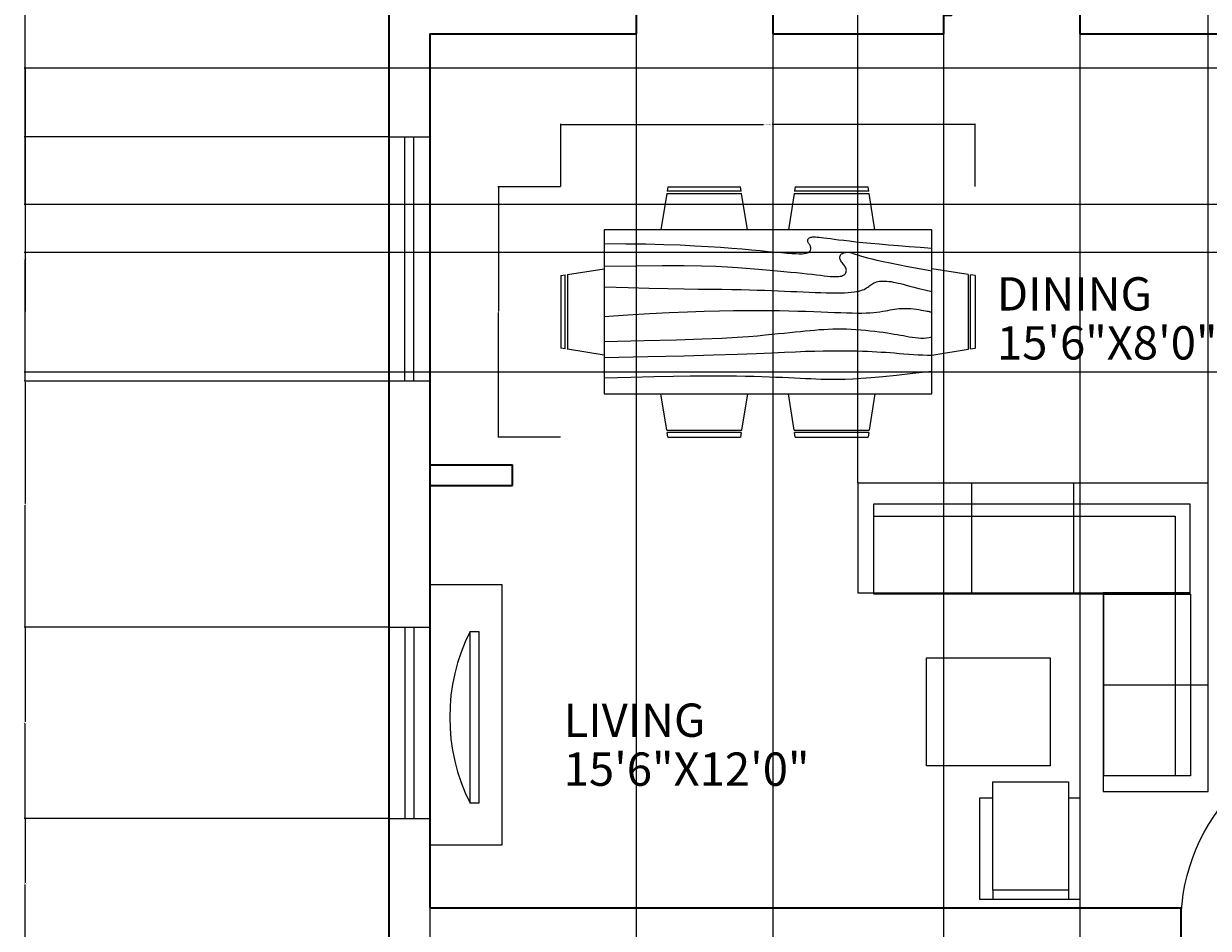
# Model space of a CAD drawing. Units: inches. Extents: x 25018 to 25490, y 41421 to 42101.
# Tile 2 of 5: x 25018 to 25279, y 41707 to 41906. Entities that reach past the tile are written whole.
import ezdxf

# ---------------------------------------------------------------- set-up
doc = ezdxf.new("R2010")
doc.units = ezdxf.units.IN
for name, color, linetype, lineweight in [('A-ANNO-DIMS', 2, 'Continuous', 18), ('A-AREA-IDEN', 7, 'Continuous', 18), ('A-DOOR', 3, 'Continuous', 25), ('A-FURN', 8, 'Continuous', 18), ('A-GLAZ', 4, 'Continuous', 18), ('A-WALL', 7, 'Continuous', 35)]:
    doc.layers.add(name, color=color, linetype=linetype, lineweight=lineweight)
doc.styles.get("Standard").update_dxf_attribs({"font": 'arial.ttf'})
doc.dimstyles.get("Standard").update_dxf_attribs({"dimtxt": 0.18, "dimasz": 0.18, "dimexe": 0.18, "dimexo": 0.0625, "dimgap": 0.09, "dimtad": 0, "dimtih": 1, "dimtoh": 1, "dimdec": 4, "dimzin": 0, "dimdsep": 46, "dimtxsty": 'Standard', "dimcen": 0.09, "dimadec": 0, "dimazin": 0, "dimtfac": 1, "dimtdec": 4, "dimtofl": 0, "dimtmove": 0, "dimatfit": 3, "dimfxl": 1, "dimtolj": 1, "dimtzin": 0, "dimarcsym": 0})

# ---------------------------------------------------------------- blocks, each defined once
blk = doc.blocks.new('*U2')
for p, q in [((0, 0), (0, -100)), ((750, 0), (750, -100))]:
    blk.add_line(p, q)
blk.add_lwpolyline([(0, 0), (0, 750), (43.75, 750), (43.75, 0)], close=True)
blk.add_arc((0, 0), 750, 0, 90)
blk = doc.blocks.new('Dining Set - 36 x 72 in.')
for p, q in [((-22, 27.5), (-22.1562, 26.50042)), ((-5.8416, 26.5), (-22.1534, 26.5)), ((-22, 27.5), (-6, 27.5)), ((-5.8437, 26.49966), (-6, 27.5)), ((6, 27.5), (5.8438, 26.50042)), ((22.1584, 26.5), (5.8466, 26.5)), ((6, 27.5), (22, 27.5)), ((22.1563, 26.49966), (22, 27.5)), ((-22.2343, 26.00059), (-23.4847, 17.99762)), ((-22.2304, 26), (-5.7608, 26)), ((-4.5152, 17.99762), (-5.7655, 25.99926)), ((5.7657, 26.00059), (4.5153, 17.99762)), ((5.7696, 26), (22.2392, 26)), ((23.4848, 17.99762), (22.2345, 25.99926)), ((36, 18), (-36, 18)), ((-36, 18), (-36, -18)), ((36, -18), (36, 18)), ((-45.5, 8), (-44.5004, 8.15617)), ((-45.5, 8), (-45.5, -8)), ((-44.5, -8.15843), (-44.5, 8.15338)), ((-44.0006, 8.23428), (-35.9976, 9.48474)), ((-44, 8.23041), (-44, -8.23915)), ((44.0006, 8.23428), (35.9976, 9.48474)), ((44, 8.23041), (44, -8.23915)), ((44.5, -8.15843), (44.5, 8.15338)), ((45.5, 8), (44.5005, 8.15617)), ((45.5, 8), (45.5, -8)), ((-44.4997, -8.15631), (-45.5, -8)), ((-35.9976, -9.48476), (-43.9993, -8.2345)), ((35.9976, -9.48476), (43.9993, -8.2345)), ((44.4997, -8.15631), (45.5, -8)), ((-36, -18), (36, -18)), ((-22.2343, -26.0006), (-23.4847, -17.99762)), ((-4.5152, -17.99762), (-5.7655, -25.99928)), ((5.7657, -26.0006), (4.5153, -17.99762)), ((23.4848, -17.99762), (22.2345, -25.99928)), ((-22.2304, -26), (-5.7608, -26)), ((5.7696, -26), (22.2392, -26)), ((-22, -27.5), (-22.1562, -26.50044)), ((-5.8416, -26.5), (-22.1534, -26.5)), ((-22, -27.5), (-6, -27.5)), ((-5.8437, -26.49967), (-6, -27.5)), ((6, -27.5), (5.8438, -26.50044)), ((22.1584, -26.5), (5.8466, -26.5)), ((6, -27.5), (22, -27.5)), ((22.1563, -26.49967), (22, -27.5))]:
    blk.add_line(p, q)
for points in [[(-36, 15), (-31.1772, 14.97754), (-26.8079, 14.91406), (-22.8538, 14.81543), (-19.276, 14.6875), (-16.0362, 14.53613), (-13.0957, 14.36718), (-10.4159, 14.18652), (-7.9583, 14), (-5.6904, 13.81315), (-3.6035, 13.63021), (-1.6954, 13.45508), (0.0365, 13.29166), (1.5945, 13.14388), (2.9811, 13.01562), (4.1988, 12.9108), (5.25, 12.83333), (6.1393, 12.78613), (6.8802, 12.76823), (7.4883, 12.77767), (7.9792, 12.8125), (8.3685, 12.87077), (8.6719, 12.95052), (8.9049, 13.0498), (9.0833, 13.16666), (9.2205, 13.29899), (9.3216, 13.44401), (9.3895, 13.59879), (9.4271, 13.76041), (9.4373, 13.92594), (9.4232, 14.09245), (9.3875, 14.257), (9.3333, 14.41666), (9.2638, 14.56917), (9.1836, 14.71484), (9.0975, 14.85465), (9.0104, 14.98958), (8.9272, 15.1206), (8.8529, 15.2487), (8.7922, 15.37483), (8.75, 15.5), (8.7305, 15.62467), (8.7344, 15.74739), (8.7617, 15.86621), (8.8125, 15.97916), (8.8867, 16.08431), (8.9844, 16.17968), (9.1055, 16.26334), (9.25, 16.33333), (9.4189, 16.38802), (9.6172, 16.42708), (9.8506, 16.45052), (10.125, 16.45833), (10.4463, 16.45052), (10.8203, 16.42708), (11.2529, 16.38802), (11.75, 16.33333), (12.3184, 16.26318), (12.9694, 16.17838), (13.7151, 16.07991), (14.5677, 15.96875), (15.5395, 15.84586), (16.6426, 15.71224), (17.8893, 15.56884), (19.2917, 15.41666), (20.859, 15.25667), (22.5879, 15.08984), (24.4721, 14.91715), (26.5052, 14.73958), (28.6809, 14.5581), (30.9929, 14.3737), (33.4347, 14.18733), (36, 14)], [(-36, 10), (-28.9766, 10.14274), (-23.1725, 10.20442), (-18.4241, 10.19775), (-14.5677, 10.13541), (-11.4399, 10.03011), (-8.877, 9.89453), (-6.7154, 9.74137), (-4.7917, 9.58333), (-2.9698, 9.43082), (-1.2246, 9.28515), (0.4415, 9.14534), (2.026, 9.01041), (3.5266, 8.87939), (4.9408, 8.7513), (6.266, 8.62516), (7.5, 8.5), (8.6411, 8.37549), (9.6914, 8.2539), (10.6538, 8.13818), (11.5312, 8.03125), (12.3267, 7.93603), (13.043, 7.85547), (13.6831, 7.79248), (14.25, 7.75), (14.7471, 7.7303), (15.1797, 7.73307), (15.5537, 7.75732), (15.875, 7.80208), (16.1494, 7.86637), (16.3828, 7.94922), (16.5811, 8.04964), (16.75, 8.16666), (16.8944, 8.29915), (17.0143, 8.44531), (17.1089, 8.60319), (17.1771, 8.77083), (17.218, 8.94629), (17.2305, 9.1276), (17.2137, 9.31282), (17.1667, 9.5), (17.0895, 9.6875), (16.987, 9.875), (16.8649, 10.0625), (16.7292, 10.25), (16.5856, 10.4375), (16.4401, 10.625), (16.2985, 10.8125), (16.1667, 11), (16.05, 11.18733), (15.9518, 11.3737), (15.8752, 11.5581), (15.8229, 11.73958), (15.798, 11.91715), (15.8034, 12.08984), (15.842, 12.25667), (15.9167, 12.41666), (16.0295, 12.56836), (16.1784, 12.70833), (16.3605, 12.83268), (16.5729, 12.9375), (16.8127, 13.01888), (17.0768, 13.07291), (17.3625, 13.0957), (17.6667, 13.08333), (17.9894, 13.03312), (18.3418, 12.94726), (18.7382, 12.82918), (19.1927, 12.68229), (19.7195, 12.51001), (20.3327, 12.31575), (21.0465, 12.10294), (21.875, 11.875), (22.8357, 11.63354), (23.959, 11.37304), (25.2786, 11.08618), (26.8282, 10.76562), (28.6414, 10.40405), (30.752, 9.99414), (33.1936, 9.52856), (36, 9)], [(-36, 5.5), (-30.7157, 5.3348), (-26.069, 5.20963), (-21.9946, 5.11767), (-18.4271, 5.05208), (-15.3009, 5.00602), (-12.5508, 4.97265), (-10.1112, 4.94515), (-7.9167, 4.91666), (-5.909, 4.88167), (-4.0586, 4.83984), (-2.3429, 4.79215), (-0.7396, 4.73958), (0.7739, 4.6831), (2.22, 4.6237), (3.6213, 4.56233), (5, 4.5), (6.373, 4.43782), (7.7344, 4.3776), (9.0723, 4.32129), (10.375, 4.27083), (11.6309, 4.22819), (12.8281, 4.19531), (13.9551, 4.17415), (15, 4.16666), (15.954, 4.17448), (16.819, 4.19791), (17.6001, 4.23698), (18.3021, 4.29166), (18.9299, 4.36198), (19.4883, 4.44791), (19.9823, 4.54948), (20.4167, 4.66666), (20.7969, 4.79899), (21.1302, 4.94401), (21.4245, 5.09879), (21.6875, 5.26041), (21.9271, 5.42594), (22.1511, 5.59245), (22.3672, 5.757), (22.5834, 5.91666), (22.8065, 6.06868), (23.0404, 6.21093), (23.2879, 6.34147), (23.5521, 6.45833), (23.8358, 6.55957), (24.142, 6.64323), (24.4735, 6.70735), (24.8334, 6.75), (25.2235, 6.76969), (25.642, 6.76692), (26.0858, 6.74267), (26.5521, 6.69791), (27.0379, 6.63362), (27.5404, 6.55078), (28.0565, 6.45036), (28.5834, 6.33333), (29.1242, 6.19987), (29.7071, 6.04687), (30.3661, 5.87044), (31.1354, 5.66666), (32.0493, 5.43164), (33.142, 5.16146), (34.4475, 4.85221), (36, 4.5)], [(-36, -1), (-30.7915, -0.6591), (-26.0195, -0.38216), (-21.6519, -0.16284), (-17.6563, 0.00521), (-14.0005, 0.12833), (-10.6523, 0.21289), (-7.5796, 0.26522), (-4.75, 0.29166), (-2.134, 0.29793), (0.2878, 0.28711), (2.5317, 0.26163), (4.6146, 0.22396), (6.5529, 0.17651), (8.3633, 0.12174), (10.0623, 0.06209), (11.6667, 0), (13.1899, -0.06201), (14.6341, -0.1211), (15.9982, -0.17432), (17.2813, -0.21875), (18.4823, -0.25147), (19.6003, -0.26953), (20.6343, -0.27002), (21.5834, -0.25), (22.4481, -0.20768), (23.2357, -0.14584), (23.9549, -0.06836), (24.6146, 0.02083), (25.2235, 0.11784), (25.7904, 0.21875), (26.3241, 0.31966), (26.8334, 0.41666), (27.3265, 0.50618), (27.8099, 0.58593), (28.2894, 0.65397), (28.7709, 0.70833), (29.2601, 0.74707), (29.763, 0.76823), (30.2855, 0.76985), (30.8334, 0.75), (31.4088, 0.70784), (31.9994, 0.64713), (32.589, 0.57275), (33.1615, 0.48958), (33.7008, 0.4025), (34.1908, 0.3164), (34.6153, 0.23616), (34.9584, 0.16666), (35.2099, 0.11165), (35.3848, 0.07031), (35.504, 0.04069), (35.5886, 0.02083), (35.6594, 0.00879), (35.7377, 0.0026), (35.8442, 0.00032), (36, 0)], [(-36, -6.5), (-27.1843, -6.31267), (-20.084, -6.1263), (-14.469, -5.9419), (-10.1094, -5.76042), (-6.7752, -5.58285), (-4.2363, -5.41016), (-2.2629, -5.24333), (-0.625, -5.08334), (0.8708, -4.93099), (2.2715, -4.78646), (3.5872, -4.64974), (4.8281, -4.52084), (6.0046, -4.39974), (7.127, -4.28646), (8.2053, -4.18099), (9.25, -4.08334), (10.2705, -3.99382), (11.2734, -3.91407), (12.2647, -3.84603), (13.25, -3.79167), (14.2354, -3.75293), (15.2266, -3.73177), (16.2295, -3.73015), (17.25, -3.75), (18.2912, -3.79248), (19.3451, -3.85547), (20.4009, -3.93604), (21.4479, -4.03125), (22.4754, -4.13819), (23.4727, -4.25391), (24.4289, -4.37549), (25.3334, -4.5), (26.1785, -4.62492), (26.9694, -4.74935), (27.7145, -4.87281), (28.4219, -4.99479), (29.1, -5.11483), (29.7572, -5.23242), (30.4016, -5.34709), (31.0417, -5.45834), (31.6837, -5.56437), (32.3262, -5.65821), (32.9658, -5.73153), (33.599, -5.77604), (34.2224, -5.78345), (34.8327, -5.74545), (35.4264, -5.65373), (36, -5.5)], [(-36, -10), (-26.4022, -9.81299), (-18.4675, -9.62891), (-11.9839, -9.45069), (-6.7396, -9.28125), (-2.5226, -9.12354), (0.8789, -8.98047), (3.6769, -8.85498), (6.0833, -8.75), (8.2767, -8.66765), (10.3021, -8.60677), (12.1712, -8.56543), (13.8958, -8.54167), (15.4876, -8.53353), (16.9583, -8.53907), (18.3197, -8.55632), (19.5834, -8.58334), (20.7616, -8.61841), (21.8685, -8.66081), (22.9188, -8.71004), (23.9271, -8.76563), (24.9081, -8.82707), (25.8763, -8.89388), (26.8465, -8.96558), (27.8334, -9.04167), (28.8474, -9.12118), (29.8828, -9.20117), (30.93, -9.27824), (31.9792, -9.34896), (33.0205, -9.40991), (34.0443, -9.45768), (35.0407, -9.48885), (36, -9.5)], [(-36, -14.5), (-30.0881, -14.33513), (-25.0332, -14.21224), (-20.7312, -14.12647), (-17.0781, -14.07292), (-13.97, -14.04671), (-11.3027, -14.04297), (-8.9724, -14.05681), (-6.875, -14.08334), (-4.9224, -14.11833), (-3.0905, -14.16016), (-1.3709, -14.20785), (0.2448, -14.26042), (1.7647, -14.3169), (3.1973, -14.3763), (4.5507, -14.43767), (5.8333, -14.5), (7.0554, -14.5621), (8.235, -14.62175), (9.3922, -14.67652), (10.5469, -14.72396), (11.7192, -14.76164), (12.929, -14.78711), (14.1965, -14.79794), (15.5417, -14.79167), (16.9933, -14.76424), (18.6152, -14.70508), (20.4804, -14.60197), (22.6615, -14.44271), (25.2312, -14.21509), (28.2624, -13.9069), (31.8277, -13.50594), (36, -13)]]:
    blk.add_lwpolyline(points)
blk = doc.blocks.new('TV-CONSOLE')
for points in [[(0, 57.27), (15.78, 57.27), (15.78, 0), (0, 0)], [(8.85, 46.95), (10.77, 46.95), (10.77, 9.28), (8.85, 9.28)]]:
    blk.add_lwpolyline(points, close=True)
blk.add_arc((46.16, 28.12), 41.8, 153.2115, 206.7885)
blk = doc.blocks.new('*D26')
at = {"layer": 'A-ANNO-DIMS', "color": 0, "lineweight": -2, "transparency": 16777216}
for p, q in [((25136.41, 41870.05), (25136.41, 41883.82)), ((25136.59, 41883.64), (25180.96, 41883.64)), ((25227.23, 41883.64), (25182.86, 41883.64)), ((25227.41, 41870.05), (25227.41, 41883.82))]:
    blk.add_line(p, q, dxfattribs=at)
at = {"layer": 'A-ANNO-DIMS', "color": 0, "transparency": 16777216}
for points in [[(25136.59, 41883.67), (25136.59, 41883.61), (25136.41, 41883.64)], [(25227.23, 41883.67), (25227.23, 41883.61), (25227.41, 41883.64)]]:
    blk.add_solid(points, dxfattribs=at)
at = {"layer": 'Defpoints', "color": 0, "transparency": 16777216}
for p in [(25227.41, 41883.64), (25136.41, 41869.99), (25227.41, 41869.99)]:
    blk.add_point(p, dxfattribs=at)
at = {"layer": 'A-ANNO-DIMS', "color": 0, "transparency": 16777216, "insert": (25181.91, 41883.64), "char_height": 0.18, "attachment_point": 5}
blk.add_mtext('\\A1;DINING SET 91', dxfattribs=at)
blk = doc.blocks.new('*D27')
at = {"layer": 'A-ANNO-DIMS', "color": 0, "lineweight": -2, "transparency": 16777216}
for p, q in [((25136.34, 41869.99), (25122.58, 41869.99)), ((25122.76, 41869.81), (25122.76, 41842.67)), ((25122.76, 41815.17), (25122.76, 41842.31)), ((25136.34, 41814.99), (25122.58, 41814.99))]:
    blk.add_line(p, q, dxfattribs=at)
at = {"layer": 'A-ANNO-DIMS', "color": 0, "transparency": 16777216}
for points in [[(25122.73, 41869.81), (25122.79, 41869.81), (25122.76, 41869.99)], [(25122.73, 41815.17), (25122.79, 41815.17), (25122.76, 41814.99)]]:
    blk.add_solid(points, dxfattribs=at)
at = {"layer": 'Defpoints', "color": 0, "transparency": 16777216}
for p in [(25122.76, 41869.99), (25136.41, 41869.99), (25136.41, 41814.99)]:
    blk.add_point(p, dxfattribs=at)
at = {"layer": 'A-ANNO-DIMS', "color": 0, "transparency": 16777216, "insert": (25122.76, 41842.49), "char_height": 0.18, "attachment_point": 5}
blk.add_mtext('\\A1;55', dxfattribs=at)
blk = doc.blocks.new('*D44')
at = {"layer": 'A-ANNO-DIMS', "color": 0, "lineweight": -2, "transparency": 16777216}
for p, q in [((25098.59, 41731.2), (25018.58, 41731.2)), ((25018.76, 41731.02), (25018.76, 41717.06)), ((25018.76, 41702.73), (25018.76, 41716.69)), ((25098.59, 41702.55), (25018.58, 41702.55))]:
    blk.add_line(p, q, dxfattribs=at)
at = {"layer": 'A-ANNO-DIMS', "color": 0, "transparency": 16777216}
for points in [[(25018.73, 41731.02), (25018.79, 41731.02), (25018.76, 41731.2)], [(25018.73, 41702.73), (25018.79, 41702.73), (25018.76, 41702.55)]]:
    blk.add_solid(points, dxfattribs=at)
at = {"layer": 'Defpoints', "color": 0, "transparency": 16777216}
for p in [(25018.76, 41731.2), (25098.65, 41731.2), (25098.65, 41702.55)]:
    blk.add_point(p, dxfattribs=at)
at = {"layer": 'A-ANNO-DIMS', "color": 0, "transparency": 16777216, "insert": (25018.76, 41716.88), "char_height": 0.18, "attachment_point": 5}
blk.add_mtext('\\A1;28.65', dxfattribs=at)
blk = doc.blocks.new('*D45')
at = {"layer": 'A-ANNO-DIMS', "color": 0, "lineweight": -2, "transparency": 16777216}
for p, q in [((25098.59, 41773.23), (25018.58, 41773.23)), ((25018.76, 41773.05), (25018.76, 41752.4)), ((25018.76, 41731.38), (25018.76, 41752.03)), ((25098.59, 41731.2), (25018.58, 41731.2))]:
    blk.add_line(p, q, dxfattribs=at)
at = {"layer": 'A-ANNO-DIMS', "color": 0, "transparency": 16777216}
for points in [[(25018.73, 41773.05), (25018.79, 41773.05), (25018.76, 41773.23)], [(25018.73, 41731.38), (25018.79, 41731.38), (25018.76, 41731.2)]]:
    blk.add_solid(points, dxfattribs=at)
at = {"layer": 'Defpoints', "color": 0, "transparency": 16777216}
for p in [(25018.76, 41773.23), (25098.65, 41773.23), (25098.65, 41731.2)]:
    blk.add_point(p, dxfattribs=at)
at = {"layer": 'A-ANNO-DIMS', "color": 0, "transparency": 16777216, "insert": (25018.76, 41752.21), "char_height": 0.18, "attachment_point": 5}
blk.add_mtext('\\A1;42.03', dxfattribs=at)
blk = doc.blocks.new('*D46')
at = {"layer": 'A-ANNO-DIMS', "color": 0, "lineweight": -2, "transparency": 16777216}
for p, q in [((25098.59, 41827.23), (25018.58, 41827.23)), ((25018.76, 41827.05), (25018.76, 41800.41)), ((25018.76, 41773.41), (25018.76, 41800.05)), ((25098.59, 41773.23), (25018.58, 41773.23))]:
    blk.add_line(p, q, dxfattribs=at)
at = {"layer": 'A-ANNO-DIMS', "color": 0, "transparency": 16777216}
for points in [[(25018.73, 41827.05), (25018.79, 41827.05), (25018.76, 41827.23)], [(25018.73, 41773.41), (25018.79, 41773.41), (25018.76, 41773.23)]]:
    blk.add_solid(points, dxfattribs=at)
at = {"layer": 'Defpoints', "color": 0, "transparency": 16777216}
for p in [(25018.76, 41827.23), (25098.65, 41827.23), (25098.65, 41773.23)]:
    blk.add_point(p, dxfattribs=at)
at = {"layer": 'A-ANNO-DIMS', "color": 0, "transparency": 16777216, "insert": (25018.76, 41800.23), "char_height": 0.18, "attachment_point": 5}
blk.add_mtext('\\A1;54', dxfattribs=at)
blk = doc.blocks.new('*D47')
at = {"layer": 'A-ANNO-DIMS', "color": 0, "lineweight": -2, "transparency": 16777216}
for p, q in [((25098.59, 41880.94), (25018.58, 41880.94)), ((25018.76, 41880.76), (25018.76, 41854.27)), ((25018.76, 41827.41), (25018.76, 41853.9)), ((25098.59, 41827.23), (25018.58, 41827.23))]:
    blk.add_line(p, q, dxfattribs=at)
at = {"layer": 'A-ANNO-DIMS', "color": 0, "transparency": 16777216}
for points in [[(25018.73, 41880.76), (25018.79, 41880.76), (25018.76, 41880.94)], [(25018.73, 41827.41), (25018.79, 41827.41), (25018.76, 41827.23)]]:
    blk.add_solid(points, dxfattribs=at)
at = {"layer": 'Defpoints', "color": 0, "transparency": 16777216}
for p in [(25018.76, 41880.94), (25098.65, 41880.94), (25098.65, 41827.23)]:
    blk.add_point(p, dxfattribs=at)
at = {"layer": 'A-ANNO-DIMS', "color": 0, "transparency": 16777216, "insert": (25018.76, 41854.09), "char_height": 0.18, "attachment_point": 5}
blk.add_mtext('\\A1;53.71', dxfattribs=at)
blk = doc.blocks.new('*D48')
at = {"layer": 'A-ANNO-DIMS', "color": 0, "lineweight": -2, "transparency": 16777216}
for p, q in [((25107.59, 42013.05), (25018.58, 42013.05)), ((25018.76, 42012.87), (25018.76, 41947.18)), ((25018.76, 41881.12), (25018.76, 41946.81)), ((25098.59, 41880.94), (25018.58, 41880.94))]:
    blk.add_line(p, q, dxfattribs=at)
at = {"layer": 'A-ANNO-DIMS', "color": 0, "transparency": 16777216}
for points in [[(25018.73, 42012.87), (25018.79, 42012.87), (25018.76, 42013.05)], [(25018.73, 41881.12), (25018.79, 41881.12), (25018.76, 41880.94)]]:
    blk.add_solid(points, dxfattribs=at)
at = {"layer": 'Defpoints', "color": 0, "transparency": 16777216}
for p in [(25018.76, 42013.05), (25107.65, 42013.05), (25098.65, 41880.94)]:
    blk.add_point(p, dxfattribs=at)
at = {"layer": 'A-ANNO-DIMS', "color": 0, "transparency": 16777216, "insert": (25018.76, 41946.99), "char_height": 0.18, "attachment_point": 5}
blk.add_mtext('\\A1;132.1', dxfattribs=at)
blk = doc.blocks.new('*D66')
at = {"layer": 'A-ANNO-DIMS', "color": 0, "lineweight": -2, "transparency": 16777216}
for p, q in [((25107.65, 41903.49), (25107.65, 41420.7)), ((25152.99, 41903.49), (25152.99, 41420.7)), ((25107.83, 41420.88), (25129.92, 41420.88)), ((25152.81, 41420.88), (25130.72, 41420.88))]:
    blk.add_line(p, q, dxfattribs=at)
at = {"layer": 'A-ANNO-DIMS', "color": 0, "transparency": 16777216}
for points in [[(25107.83, 41420.91), (25107.83, 41420.85), (25107.65, 41420.88)], [(25152.81, 41420.91), (25152.81, 41420.85), (25152.99, 41420.88)]]:
    blk.add_solid(points, dxfattribs=at)
at = {"layer": 'Defpoints', "color": 0, "transparency": 16777216}
for p in [(25107.65, 41903.55), (25152.99, 41903.55), (25152.99, 41420.88)]:
    blk.add_point(p, dxfattribs=at)
at = {"layer": 'A-ANNO-DIMS', "color": 0, "transparency": 16777216, "insert": (25130.32, 41420.88), "char_height": 0.18, "attachment_point": 5}
blk.add_mtext('\\A1;45.34', dxfattribs=at)
blk = doc.blocks.new('*D67')
at = {"layer": 'A-ANNO-DIMS', "color": 0, "lineweight": -2, "transparency": 16777216}
for p, q in [((25152.99, 41903.49), (25152.99, 41420.7)), ((25182.99, 41903.49), (25182.99, 41420.7)), ((25153.17, 41420.88), (25167.77, 41420.88)), ((25182.81, 41420.88), (25168.21, 41420.88))]:
    blk.add_line(p, q, dxfattribs=at)
at = {"layer": 'A-ANNO-DIMS', "color": 0, "transparency": 16777216}
for points in [[(25153.17, 41420.91), (25153.17, 41420.85), (25152.99, 41420.88)], [(25182.81, 41420.91), (25182.81, 41420.85), (25182.99, 41420.88)]]:
    blk.add_solid(points, dxfattribs=at)
at = {"layer": 'Defpoints', "color": 0, "transparency": 16777216}
for p in [(25152.99, 41903.55), (25182.99, 41903.55), (25182.99, 41420.88)]:
    blk.add_point(p, dxfattribs=at)
at = {"layer": 'A-ANNO-DIMS', "color": 0, "transparency": 16777216, "insert": (25167.99, 41420.88), "char_height": 0.18, "attachment_point": 5}
blk.add_mtext('\\A1;30', dxfattribs=at)
blk = doc.blocks.new('*D68')
at = {"layer": 'A-ANNO-DIMS', "color": 0, "lineweight": -2, "transparency": 16777216}
for p, q in [((25182.99, 41903.49), (25182.99, 41420.7)), ((25220.45, 41903.49), (25220.45, 41420.7)), ((25183.17, 41420.88), (25201.26, 41420.88)), ((25220.27, 41420.88), (25202.18, 41420.88))]:
    blk.add_line(p, q, dxfattribs=at)
at = {"layer": 'A-ANNO-DIMS', "color": 0, "transparency": 16777216}
for points in [[(25183.17, 41420.91), (25183.17, 41420.85), (25182.99, 41420.88)], [(25220.27, 41420.91), (25220.27, 41420.85), (25220.45, 41420.88)]]:
    blk.add_solid(points, dxfattribs=at)
at = {"layer": 'Defpoints', "color": 0, "transparency": 16777216}
for p in [(25182.99, 41903.55), (25220.45, 41903.55), (25220.45, 41420.88)]:
    blk.add_point(p, dxfattribs=at)
at = {"layer": 'A-ANNO-DIMS', "color": 0, "transparency": 16777216, "insert": (25201.72, 41420.88), "char_height": 0.18, "attachment_point": 5}
blk.add_mtext('\\A1;37.464', dxfattribs=at)
blk = doc.blocks.new('*D69')
at = {"layer": 'A-ANNO-DIMS', "color": 0, "lineweight": -2, "transparency": 16777216}
for p, q in [((25220.45, 41903.49), (25220.45, 41420.7)), ((25250.45, 41903.49), (25250.45, 41420.7)), ((25220.63, 41420.88), (25235.23, 41420.88)), ((25250.27, 41420.88), (25235.67, 41420.88))]:
    blk.add_line(p, q, dxfattribs=at)
at = {"layer": 'A-ANNO-DIMS', "color": 0, "transparency": 16777216}
for points in [[(25220.63, 41420.91), (25220.63, 41420.85), (25220.45, 41420.88)], [(25250.27, 41420.91), (25250.27, 41420.85), (25250.45, 41420.88)]]:
    blk.add_solid(points, dxfattribs=at)
at = {"layer": 'Defpoints', "color": 0, "transparency": 16777216}
for p in [(25220.45, 41903.55), (25250.45, 41903.55), (25250.45, 41420.88)]:
    blk.add_point(p, dxfattribs=at)
at = {"layer": 'A-ANNO-DIMS', "color": 0, "transparency": 16777216, "insert": (25235.45, 41420.88), "char_height": 0.18, "attachment_point": 5}
blk.add_mtext('\\A1;30', dxfattribs=at)
blk = doc.blocks.new('*D70')
at = {"layer": 'A-ANNO-DIMS', "color": 0, "lineweight": -2, "transparency": 16777216}
for p, q in [((25250.45, 41903.49), (25250.45, 41420.7)), ((25302.95, 41903.49), (25302.95, 41420.7)), ((25250.63, 41420.88), (25276.38, 41420.88)), ((25302.77, 41420.88), (25277.03, 41420.88))]:
    blk.add_line(p, q, dxfattribs=at)
at = {"layer": 'A-ANNO-DIMS', "color": 0, "transparency": 16777216}
for points in [[(25250.63, 41420.91), (25250.63, 41420.85), (25250.45, 41420.88)], [(25302.77, 41420.91), (25302.77, 41420.85), (25302.95, 41420.88)]]:
    blk.add_solid(points, dxfattribs=at)
at = {"layer": 'Defpoints', "color": 0, "transparency": 16777216}
for p in [(25250.45, 41903.55), (25302.95, 41903.55), (25302.95, 41420.88)]:
    blk.add_point(p, dxfattribs=at)
at = {"layer": 'A-ANNO-DIMS', "color": 0, "transparency": 16777216, "insert": (25276.7, 41420.88), "char_height": 0.18, "attachment_point": 5}
blk.add_mtext('\\A1;52.5', dxfattribs=at)
blk = doc.blocks.new('*D72')
at = {"layer": 'A-ANNO-DIMS', "color": 0, "lineweight": -2, "transparency": 16777216}
for p, q in [((25338.89, 41896.05), (25018.58, 41896.05)), ((25018.76, 41895.87), (25018.76, 41881.23)), ((25018.76, 41866.23), (25018.76, 41880.87)), ((25338.89, 41866.05), (25018.58, 41866.05))]:
    blk.add_line(p, q, dxfattribs=at)
at = {"layer": 'A-ANNO-DIMS', "color": 0, "transparency": 16777216}
for points in [[(25018.73, 41895.87), (25018.79, 41895.87), (25018.76, 41896.05)], [(25018.73, 41866.23), (25018.79, 41866.23), (25018.76, 41866.05)]]:
    blk.add_solid(points, dxfattribs=at)
at = {"layer": 'Defpoints', "color": 0, "transparency": 16777216}
for p in [(25018.76, 41896.05), (25338.95, 41896.05), (25338.95, 41866.05)]:
    blk.add_point(p, dxfattribs=at)
at = {"layer": 'A-ANNO-DIMS', "color": 0, "transparency": 16777216, "insert": (25018.76, 41881.05), "char_height": 0.18, "attachment_point": 5}
blk.add_mtext('\\A1;30', dxfattribs=at)
blk = doc.blocks.new('*D73')
at = {"layer": 'A-ANNO-DIMS', "color": 0, "lineweight": -2, "transparency": 16777216}
for p, q in [((25338.89, 41855.55), (25018.58, 41855.55)), ((25018.76, 41855.37), (25018.76, 41842.58)), ((25018.76, 41829.43), (25018.76, 41842.22)), ((25338.89, 41829.25), (25018.58, 41829.25))]:
    blk.add_line(p, q, dxfattribs=at)
at = {"layer": 'A-ANNO-DIMS', "color": 0, "transparency": 16777216}
for points in [[(25018.73, 41855.37), (25018.79, 41855.37), (25018.76, 41855.55)], [(25018.73, 41829.43), (25018.79, 41829.43), (25018.76, 41829.25)]]:
    blk.add_solid(points, dxfattribs=at)
at = {"layer": 'Defpoints', "color": 0, "transparency": 16777216}
for p in [(25018.76, 41855.55), (25338.95, 41855.55), (25338.95, 41829.25)]:
    blk.add_point(p, dxfattribs=at)
at = {"layer": 'A-ANNO-DIMS', "color": 0, "transparency": 16777216, "insert": (25018.76, 41842.4), "char_height": 0.18, "attachment_point": 5}
blk.add_mtext('\\A1;26.3', dxfattribs=at)
blk = doc.blocks.new('*D75')
at = {"layer": 'A-ANNO-DIMS', "color": 0, "lineweight": -2, "transparency": 16777216}
for p, q in [((25201.64, 41804.94), (25201.64, 42101.23)), ((25201.82, 42101.05), (25239.92, 42101.05)), ((25278.45, 42101.05), (25240.36, 42101.05)), ((25278.63, 41804.94), (25278.63, 42101.23))]:
    blk.add_line(p, q, dxfattribs=at)
at = {"layer": 'A-ANNO-DIMS', "color": 0, "transparency": 16777216}
for points in [[(25201.82, 42101.08), (25201.82, 42101.02), (25201.64, 42101.05)], [(25278.45, 42101.08), (25278.45, 42101.02), (25278.63, 42101.05)]]:
    blk.add_solid(points, dxfattribs=at)
at = {"layer": 'Defpoints', "color": 0, "transparency": 16777216}
for p in [(25278.63, 42101.05), (25201.64, 41804.88), (25278.63, 41804.88)]:
    blk.add_point(p, dxfattribs=at)
at = {"layer": 'A-ANNO-DIMS', "color": 0, "transparency": 16777216, "insert": (25240.14, 42101.05), "char_height": 0.18, "attachment_point": 5}
blk.add_mtext('\\A1;77', dxfattribs=at)

msp = doc.modelspace()

# ---------------------------------------------------------------- linework, layer by layer
at = {"layer": 'A-FURN'}
for p, q in [((25226.6989, 41780.4798), (25226.6989, 41804.8791)), ((25249.072, 41780.7463), (25249.072, 41804.8791)), ((25205.1776, 41797.5732), (25271.3505, 41797.5732)), ((25271.3505, 41797.5732), (25271.3505, 41740.5726)), ((25255.6714, 41760.5262), (25278.6341, 41760.5262)), ((25231.3361, 41715.4665), (25231.3361, 41713.3629)), ((25247.8933, 41715.4665), (25247.8933, 41713.3629))]:
    msp.add_line(p, q, dxfattribs=at)
for points in [[(25278.6341, 41780.7463), (25278.6341, 41804.8791), (25201.6418, 41804.8791), (25201.6418, 41780.7463), (25274.5613, 41780.7463)], [(25274.5613, 41780.7463), (25255.5493, 41780.7463), (25255.5493, 41737.1033), (25278.6341, 41737.1033), (25278.6341, 41780.7463)], [(25247.8933, 41735.7013), (25250.4511, 41735.7013), (25250.4511, 41713.3629), (25228.4738, 41713.3629), (25228.4738, 41735.7013), (25231.3361, 41735.7013)]]:
    msp.add_lwpolyline(points, dxfattribs=at)
for points in [[(25205.1776, 41800.3259), (25274.5613, 41800.3259), (25274.5613, 41780.4798), (25205.1776, 41780.4798)], [(25255.6714, 41780.4798), (25274.7316, 41780.4798), (25274.7316, 41740.5726), (25255.6714, 41740.5726)], [(25216.7422, 41766.4813), (25243.865, 41766.4813), (25243.865, 41742.7364), (25216.7422, 41742.7364)], [(25231.3361, 41739.2219), (25247.8933, 41739.2219), (25247.8933, 41715.4665), (25231.3361, 41715.4665)]]:
    msp.add_lwpolyline(points, close=True, dxfattribs=at)
at = {"layer": 'A-GLAZ'}
for p, q in [((25098.6526, 41880.9383), (25107.6526, 41880.9383)), ((25102.1526, 41827.2319), (25102.1526, 41880.9383)), ((25104.1526, 41827.2319), (25104.1526, 41880.9383)), ((25107.6526, 41827.2319), (25098.6526, 41827.2319)), ((25098.6526, 41773.2272), (25107.6526, 41773.2272)), ((25102.1526, 41773.2272), (25102.1526, 41731.2013)), ((25104.1526, 41773.2272), (25104.1526, 41731.2013)), ((25098.6526, 41731.2013), (25107.6526, 41731.2013))]:
    msp.add_line(p, q, dxfattribs=at)
at = {"layer": 'A-WALL'}
for p, q in [((25098.6526, 42070.0498), (25098.6526, 41501.5498)), ((25152.9888, 41908.0498), (25152.9888, 41903.5498)), ((25182.9888, 41908.0498), (25182.9888, 41903.5498)), ((25220.4527, 41908.0498), (25220.4527, 41903.5498)), ((25250.4527, 41908.0498), (25250.4527, 41903.5498)), ((25107.6526, 41903.5498), (25152.9888, 41903.5498)), ((25107.6526, 41903.5498), (25107.6526, 41711.5498)), ((25182.9888, 41903.5498), (25220.4527, 41903.5498)), ((25250.4527, 41903.5498), (25302.9527, 41903.5498)), ((25107.6526, 41808.8674), (25125.7953, 41808.8674)), ((25125.7953, 41804.3674), (25125.7953, 41808.8674)), ((25107.6526, 41804.3674), (25125.7953, 41804.3674)), ((25107.6526, 41711.5498), (25272.6526, 41711.5498)), ((25272.6526, 41702.5498), (25272.6526, 41711.5498))]:
    msp.add_line(p, q, dxfattribs=at)

# ---------------------------------------------------------------- block references
at = {"layer": 'A-DOOR'}
for p, xscale, yscale, zscale in [((25220.4527, 41907.5498), 0.0400000000000011, 0.0400000000000011, 0.0400000000000011), ((25314.6526, 41708.1498), -0.0560000000000015, 0.0560000000000015, 0.0560000000000015)]:
    msp.add_blockref('*U2', p, dxfattribs=dict(at, xscale=xscale, yscale=yscale, zscale=zscale))
at = {"layer": 'A-FURN'}
for name, p in [('Dining Set - 36 x 72 in.', (25181.9074, 41842.4911)), ('TV-CONSOLE', (25107.653, 41725.296))]:
    msp.add_blockref(name, p, dxfattribs=at)

# ---------------------------------------------------------------- texts
at = {"layer": 'A-AREA-IDEN'}
for s, height, p in [('DINING', 7.32047, (25232.1929, 41842.7786)), ('15\'6"X8\'0"', 7.32047, (25232.2006, 41832.0193)), ('LIVING', 7.32047, (25137.0392, 41749.1187)), ('15\'6"X12\'0"', 7.320471, (25137.0468, 41738.3594))]:
    msp.add_text(s, height=height, dxfattribs=at).set_placement(p)

# ---------------------------------------------------------------- dimensions: what is measured, and where the dimension line sits
at = {"layer": 'A-ANNO-DIMS'}
for base, p1, p2, override, picture, middle in [((25278.6341, 42101.0498), (25201.6418, 41804.8791), (25278.6341, 41804.8791), {"dimdec": 0, "dimlfac": 1, "dimrnd": 0, "dimzin": 0, "dimdsep": 46, "dimlunit": 2}, '*D75', (25240.138, 42101.0498)), ((25152.9888, 41420.8835), (25107.6526, 41903.5498), (25152.9888, 41903.5498), {"dimdec": 2, "dimlfac": 1, "dimrnd": 0, "dimzin": 0, "dimdsep": 46, "dimlunit": 2}, '*D66', (25130.3207, 41420.8835)), ((25182.9888, 41420.8835), (25152.9888, 41903.5498), (25182.9888, 41903.5498), {"dimdec": 0, "dimlfac": 1, "dimrnd": 0, "dimzin": 0, "dimdsep": 46, "dimlunit": 2}, '*D67', (25167.9888, 41420.8835)), ((25220.4527, 41420.8835), (25182.9888, 41903.5498), (25220.4527, 41903.5498), {"dimdec": 3, "dimlfac": 1, "dimrnd": 0, "dimzin": 0, "dimdsep": 46, "dimlunit": 2}, '*D68', (25201.7208, 41420.8835)), ((25250.4527, 41420.8835), (25220.4527, 41903.5498), (25250.4527, 41903.5498), {"dimdec": 0, "dimlfac": 1, "dimrnd": 0, "dimzin": 0, "dimdsep": 46, "dimlunit": 2}, '*D69', (25235.4527, 41420.8835)), ((25302.9527, 41420.8835), (25250.4527, 41903.5498), (25302.9527, 41903.5498), {"dimdec": 1, "dimlfac": 1, "dimrnd": 0, "dimzin": 0, "dimdsep": 46, "dimlunit": 2}, '*D70', (25276.7027, 41420.8835))]:
    dim = msp.add_linear_dim(base=base, p1=p1, p2=p2, dimstyle='Standard', override=override, dxfattribs=at)
    dim.commit()
    dim.dimension.update_dxf_attribs({"geometry": picture, "text_midpoint": middle})
for base, p1, p2, override, picture, middle in [((25018.7568, 42013.0498), (25098.6526, 41880.9383), (25107.6526, 42013.0498), {"dimdec": 1, "dimlfac": 1, "dimrnd": 0, "dimzin": 0, "dimdsep": 46, "dimlunit": 2}, '*D48', (25018.7568, 41946.994)), ((25018.7568, 41896.0498), (25338.9527, 41866.0498), (25338.9527, 41896.0498), {"dimdec": 0, "dimlfac": 1, "dimrnd": 0, "dimzin": 0, "dimdsep": 46, "dimlunit": 2}, '*D72', (25018.7568, 41881.0498)), ((25018.7568, 41880.9383), (25098.6526, 41827.2319), (25098.6526, 41880.9383), {"dimdec": 2, "dimlfac": 1, "dimrnd": 0, "dimzin": 0, "dimdsep": 46, "dimlunit": 2}, '*D47', (25018.7568, 41854.0851)), ((25122.7574, 41869.9911), (25136.4074, 41814.9911), (25136.4074, 41869.9911), {"dimdec": 0, "dimlfac": 1, "dimrnd": 0, "dimzin": 0, "dimdsep": 46, "dimlunit": 2}, '*D27', (25122.7574, 41842.4911)), ((25018.7568, 41855.5498), (25338.9527, 41829.2485), (25338.9527, 41855.5498), {"dimdec": 1, "dimlfac": 1, "dimrnd": 0, "dimzin": 0, "dimdsep": 46, "dimlunit": 2}, '*D73', (25018.7568, 41842.3992)), ((25018.7568, 41827.2319), (25098.6526, 41773.2272), (25098.6526, 41827.2319), {"dimdec": 0, "dimlfac": 1, "dimrnd": 0, "dimzin": 0, "dimdsep": 46, "dimlunit": 2}, '*D46', (25018.7568, 41800.2295)), ((25018.7568, 41773.2272), (25098.6526, 41731.2013), (25098.6526, 41773.2272), {"dimdec": 2, "dimlfac": 1, "dimrnd": 0, "dimzin": 0, "dimdsep": 46, "dimlunit": 2}, '*D45', (25018.7568, 41752.2143)), ((25018.7568, 41731.2013), (25098.6526, 41702.5498), (25098.6526, 41731.2013), {"dimdec": 2, "dimlfac": 1, "dimrnd": 0, "dimzin": 0, "dimdsep": 46, "dimlunit": 2}, '*D44', (25018.7568, 41716.8756))]:
    dim = msp.add_linear_dim(base=base, p1=p1, p2=p2, angle=90, dimstyle='Standard', override=override, dxfattribs=at)
    dim.commit()
    dim.dimension.update_dxf_attribs({"geometry": picture, "text_midpoint": middle})
dim = msp.add_linear_dim(base=(25227.4074, 41883.6411), p1=(25136.4074, 41869.9911), p2=(25227.4074, 41869.9911), text='DINING SET <>', dimstyle='Standard', override={"dimdec": 0, "dimlfac": 1, "dimrnd": 0, "dimzin": 0, "dimdsep": 46, "dimlunit": 2}, dxfattribs=at)
dim.commit()
dim.dimension.update_dxf_attribs({"geometry": '*D26', "text_midpoint": (25181.9074, 41883.6411)})

doc.saveas('drawing.dxf')
